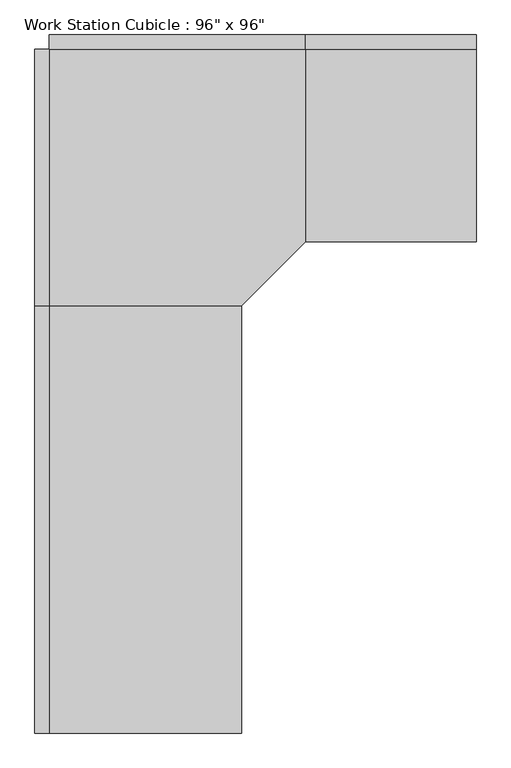
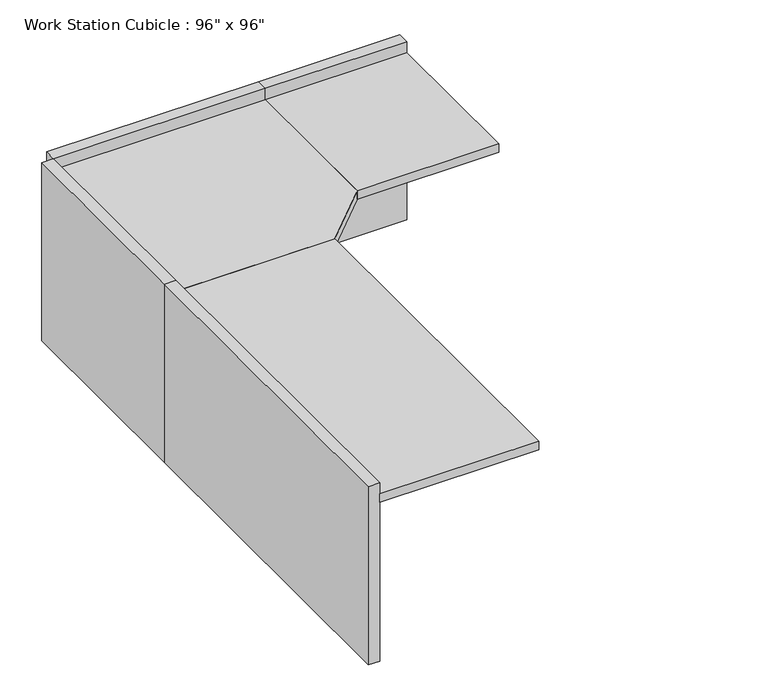
"""IFC4 building model written with IfcOpenShell, lengths in millimetres: furniture geometry."""

from ifc_helpers import new_model, si_unit, frame, origin, origin_with_axes, place, context, project, spatial, polyline, outline, extrude, source, transform, mapped, element, save


def furniture_a415b6c7(model_context):
    return source(origin(), model_context, "Body", "SweptSolid", [
        extrude(outline(polyline([(-80.9317522, -545.8230076), (833.4682478, -545.8230076), (833.4682478, -1231.6230076), (604.8682478, -1460.2230076), (-80.9317522, -1460.2230076), (-80.9317522, -545.8230076)])), frame((0.0, 0.0, 723.9), z_axis=(0.0, 0.0, 1.0), x_axis=(1.0, 0.0, 0.0)), (0.0, 0.0, 1.0), 38.1),
        extrude(outline(polyline([(604.8682478, -2984.2230076), (-80.9317522, -2984.2230076), (-80.9317522, -1460.2230076), (604.8682478, -1460.2230076), (604.8682478, -2984.2230076)])), frame((0.0, 0.0, 723.9), z_axis=(0.0, 0.0, 1.0), x_axis=(1.0, 0.0, 0.0)), (0.0, 0.0, 1.0), 38.1),
        extrude(outline(polyline([(1443.0682478, -1231.6230076), (833.4682478, -1231.6230076), (833.4682478, -545.8230076), (1443.0682478, -545.8230076), (1443.0682478, -1231.6230076)])), frame((0.0, 0.0, 723.9), z_axis=(0.0, 0.0, 1.0), x_axis=(1.0, 0.0, 0.0)), (0.0, 0.0, 1.0), 38.1),
        extrude(outline(polyline([(1443.0682478, -545.8230076), (833.4682478, -545.8230076), (833.4682478, -495.0230076), (1443.0682478, -495.0230076), (1443.0682478, -545.8230076)])), origin_with_axes(), (0.0, 0.0, 1.0), 812.8),
        extrude(outline(polyline([(833.4682478, -545.8230076), (-80.9317522, -545.8230076), (-80.9317522, -495.0230076), (833.4682478, -495.0230076), (833.4682478, -545.8230076)])), origin_with_axes(), (0.0, 0.0, 1.0), 812.8),
        extrude(outline(polyline([(-80.9317522, -1460.2230076), (-131.7317522, -1460.2230076), (-131.7317522, -545.8230076), (-80.9317522, -545.8230076), (-80.9317522, -1460.2230076)])), origin_with_axes(), (0.0, 0.0, 1.0), 812.8),
        extrude(outline(polyline([(-80.9317522, -2984.2230076), (-131.7317522, -2984.2230076), (-131.7317522, -1460.2230076), (-80.9317522, -1460.2230076), (-80.9317522, -2984.2230076)])), origin_with_axes(), (0.0, 0.0, 1.0), 812.8),
    ])


if __name__ == "__main__":
    model = new_model("IFC4")
    model_context = context("Model", 3, world=origin())
    ifc_project = project(units=[si_unit("LENGTHUNIT", "METRE", prefix="MILLI")], contexts=[model_context])
    site = spatial("IfcSite", under=ifc_project)
    building = spatial("IfcBuilding", under=site)
    placement = place(None, origin())
    furniture_shape = furniture_a415b6c7(model_context)
    element("IfcFurniture", 1, ObjectType="Work Station Cubicle : 96\" x 96\"", at=placement, inside=building, context=model_context, shape_type="MappedRepresentation", body=[
        mapped(furniture_shape, transform((0.0, 0.0, 0.0), x_axis=(1.0, 0.0, 0.0), y_axis=(0.0, 1.0, 0.0), z_axis=(0.0, 0.0, 1.0))),
    ])
    save(model, "model.ifc")

# Revit data of these elements
# Type "Work Station Cubicle : 96\" x 96\""
#   Assembly Code = "E2020"
#   Desktop Height = 2' - 6"
#   Desktop1 Width = 2' - 3"
#   Desktop2 Width = 2' - 3"
#   Panel Height = 2' - 8"
#   Panel1 Length = 5' - 0"
#   Panel2 Length = 2' - 0"
#   Cube Panel Material = Textile - Light Gray
#   Work Top Material = Laminate, Ivory, Matte
#   Default Elevation = 0
# Element 1 (IfcFurniture, "Work Station Cubicle : 96\" x 96\"")
#   Materials on its faces: "Textile - Light Gray", "Laminate, Ivory, Matte"
# Materials
#   "Textile - Light Gray": class "Fabric", colour RGB 204 204 204, transparency 0
#   "Laminate, Ivory, Matte": class "Plastic", colour RGB 247 247 239, transparency 0, Description = "Plastic Laminate - Ivory, Matte", Cost = 0
